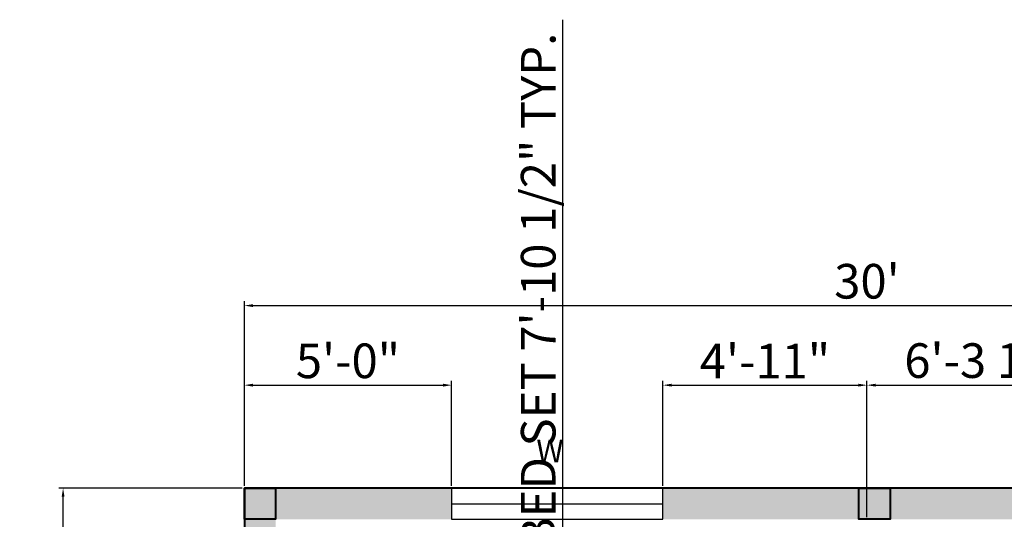
# Model space of a CAD drawing. Units: inches. Extents: x 1628 to 2197, y 2073 to 2736.
# Tile 2 of 3: x 1628 to 1913, y 2592 to 2736. Entities that reach past the tile are written whole.
import ezdxf

# ---------------------------------------------------------------- set-up
doc = ezdxf.new("R2010")
doc.units = ezdxf.units.IN
for name, color, linetype, lineweight in [('A-ANNO-DIMS', 2, 'Continuous', 18), ('A-ANNO-IDEN', 7, 'Continuous', 18), ('A-COLS', 7, 'Continuous', 40), ('A-COLS-PATT', 8, 'Continuous', 13), ('A-WALL-PATT', 152, 'Continuous', 13), ('wall', 151, 'Continuous', 40), ('window', 20, 'Continuous', 25)]:
    doc.layers.add(name, color=color, linetype=linetype, lineweight=lineweight)
doc.styles.get("Standard").update_dxf_attribs({"font": 'arial.ttf'})
doc.dimstyles.new('ISO-25', dxfattribs={"dimtxt": 10, "dimasz": 2.5, "dimexe": 1.25, "dimexo": 0.625, "dimtad": 1, "dimdec": 0, "dimlunit": 4, "dimtxsty": 'Standard', "dimcen": 2.5, "dimadec": 0, "dimazin": 0, "dimtfac": 1, "dimtdec": 0, "dimtmove": 0, "dimatfit": 3, "dimfxl": 1, "dimarcsym": 0})

# ---------------------------------------------------------------- blocks, each defined once
blk = doc.blocks.new('*D5')
at = {"layer": 'A-ANNO-DIMS', "color": 0, "lineweight": -2, "transparency": 16777216}
for p, q in [((1693.110896843685, 2601.327398616903), (1693.110896843685, 2654.686150997897)), ((1695.610896843685, 2653.436150997897), (2050.610896843686, 2653.436150997897)), ((2053.110896843686, 2601.327398616903), (2053.110896843686, 2654.686150997897))]:
    blk.add_line(p, q, dxfattribs=at)
at = {"layer": 'A-ANNO-DIMS', "color": 0, "transparency": 16777216}
for points in [[(1695.610896843685, 2653.852817664564), (1695.610896843685, 2653.019484331231), (1693.110896843685, 2653.436150997897)], [(2050.610896843686, 2653.852817664564), (2050.610896843686, 2653.019484331231), (2053.110896843686, 2653.436150997897)]]:
    blk.add_solid(points, dxfattribs=at)
at = {"layer": 'Defpoints', "color": 0, "transparency": 16777216}
for p in [(2053.110896843686, 2653.436150997897), (1693.110896843685, 2600.702398616903), (2053.110896843686, 2600.702398616903)]:
    blk.add_point(p, dxfattribs=at)
at = {"layer": 'A-ANNO-DIMS', "color": 0, "transparency": 16777216, "insert": (1873.110896843686, 2659.170291516315), "char_height": 10, "attachment_point": 5}
blk.add_mtext("30'", dxfattribs=at)
blk = doc.blocks.new('*D6')
at = {"layer": 'A-ANNO-DIMS', "color": 0, "lineweight": -2, "transparency": 16777216}
for p, q in [((1692.485896843686, 2600.702398616904), (1639.445355811252, 2600.702398616904)), ((1640.695355811253, 2123.202398616904), (1640.695355811252, 2598.202398616904)), ((1692.485896843686, 2120.702398616904), (1639.445355811253, 2120.702398616904))]:
    blk.add_line(p, q, dxfattribs=at)
at = {"layer": 'A-ANNO-DIMS', "color": 0, "transparency": 16777216}
for points in [[(1640.278689144586, 2598.202398616904), (1641.112022477919, 2598.202398616904), (1640.695355811252, 2600.702398616904)], [(1640.278689144586, 2123.202398616904), (1641.112022477919, 2123.202398616904), (1640.695355811253, 2120.702398616904)]]:
    blk.add_solid(points, dxfattribs=at)
at = {"layer": 'Defpoints', "color": 0, "transparency": 16777216}
for p in [(1640.695355811252, 2600.702398616904), (1693.110896843687, 2600.702398616904), (1693.110896843687, 2120.702398616904)]:
    blk.add_point(p, dxfattribs=at)
at = {"layer": 'A-ANNO-DIMS', "color": 0, "transparency": 16777216, "insert": (1634.964625934036, 2360.702398616903), "char_height": 10, "attachment_point": 5, "rotation": 90}
blk.add_mtext("40'", dxfattribs=at)
blk = doc.blocks.new('WINDOW-61IN')
blk.add_line((-0.0003684333103138, 4.500398616903112), (61.10273973038352, 4.500398616903112))
blk.add_lwpolyline([(-0.0003684333103138, 0.0003986169031123), (61.10273973038352, 0.0003986169031123), (61.10273973038352, 9.000398616903112), (-0.0003684333103138, 9.000398616903112)], close=True)
blk = doc.blocks.new('COLUMN-9X9')
blk.add_lwpolyline([(-0.0001031563144807, 9.000398616903112), (8.99989684368552, 9.000398616903112), (8.99989684368552, 0.0003986169031123), (-0.0001031563144807, 0.0003986169031123)], close=True)
blk = doc.blocks.new('*D19')
at = {"layer": 'A-ANNO-DIMS', "color": 0, "lineweight": -2, "transparency": 16777216}
for p, q in [((1785.152754647198, 2577.035625777927), (1785.152754647198, 2736.024370661965)), ((1771.578393576364, 2577.035625777927), (1786.402754647198, 2577.035625777927)), ((1785.152754647198, 2484.873218639036), (1785.152754647198, 2574.535625777927)), ((1771.578393576364, 2482.373218639037), (1786.402754647198, 2482.373218639037))]:
    blk.add_line(p, q, dxfattribs=at)
at = {"layer": 'A-ANNO-DIMS', "color": 0, "transparency": 16777216}
for points in [[(1784.736087980531, 2574.535625777927), (1785.569421313865, 2574.535625777927), (1785.152754647198, 2577.035625777927)], [(1784.736087980532, 2484.873218639036), (1785.569421313865, 2484.873218639036), (1785.152754647198, 2482.373218639037)]]:
    blk.add_solid(points, dxfattribs=at)
at = {"layer": 'Defpoints', "color": 0, "transparency": 16777216}
for p in [(1770.953393576364, 2577.035625777927), (1785.152754647198, 2577.035625777927), (1770.953393576364, 2482.373218639037)]:
    blk.add_point(p, dxfattribs=at)
at = {"layer": 'A-ANNO-DIMS', "color": 0, "transparency": 16777216, "insert": (1779.357222587171, 2657.779998219945), "char_height": 10, "attachment_point": 5, "rotation": 90}
blk.add_mtext('BED SET 7\'-10 1/2" TYP.', dxfattribs=at)
blk = doc.blocks.new('*D25')
at = {"layer": 'A-ANNO-DIMS', "color": 0, "lineweight": -2, "transparency": 16777216}
for p, q in [((1693.110897, 2601.327399), (1693.110897, 2631.702399)), ((1695.610897, 2630.452399), (1750.513632, 2630.452399)), ((1753.013632, 2601.327399), (1753.013632, 2631.702399))]:
    blk.add_line(p, q, dxfattribs=at)
at = {"layer": 'A-ANNO-DIMS', "color": 0, "transparency": 16777216}
for points in [[(1695.610897, 2630.869065666666), (1695.610897, 2630.035732333333), (1693.110897, 2630.452399)], [(1750.513632, 2630.869065666666), (1750.513632, 2630.035732333333), (1753.013632, 2630.452399)]]:
    blk.add_solid(points, dxfattribs=at)
at = {"layer": 'Defpoints', "color": 0, "transparency": 16777216}
for p in [(1753.013632, 2630.452399), (1693.110897, 2600.702399), (1753.013632, 2600.702399)]:
    blk.add_point(p, dxfattribs=at)
at = {"layer": 'A-ANNO-DIMS', "color": 0, "transparency": 16777216, "insert": (1723.0622645, 2636.183128877217), "char_height": 10, "attachment_point": 5}
blk.add_mtext('5\'-0"', dxfattribs=at)
blk = doc.blocks.new('*D26')
at = {"layer": 'A-ANNO-DIMS', "color": 0, "lineweight": -2, "transparency": 16777216}
for p, q in [((1814.11674, 2601.327399), (1814.11674, 2631.702399)), ((1816.61674, 2630.452399), (1870.610897, 2630.452399)), ((1873.110897, 2592.327399), (1873.110897, 2631.702399))]:
    blk.add_line(p, q, dxfattribs=at)
at = {"layer": 'A-ANNO-DIMS', "color": 0, "transparency": 16777216}
for points in [[(1816.61674, 2630.869065666666), (1816.61674, 2630.035732333333), (1814.11674, 2630.452399)], [(1870.610897, 2630.869065666666), (1870.610897, 2630.035732333333), (1873.110897, 2630.452399)]]:
    blk.add_solid(points, dxfattribs=at)
at = {"layer": 'Defpoints', "color": 0, "transparency": 16777216}
for p in [(1873.110897, 2630.452399), (1814.11674, 2600.702399), (1873.110897, 2591.702399)]:
    blk.add_point(p, dxfattribs=at)
at = {"layer": 'A-ANNO-DIMS', "color": 0, "transparency": 16777216, "insert": (1843.6138185, 2636.097862847203), "char_height": 10, "attachment_point": 5}
blk.add_mtext('4\'-11"', dxfattribs=at)
blk = doc.blocks.new('*D27')
at = {"layer": 'A-ANNO-DIMS', "color": 0, "lineweight": -2, "transparency": 16777216}
for p, q in [((1873.110897, 2592.327399), (1873.110897, 2631.702399)), ((1875.610897, 2630.452399), (1945.868746, 2630.452399)), ((1948.368746, 2601.327399), (1948.368746, 2631.702399))]:
    blk.add_line(p, q, dxfattribs=at)
at = {"layer": 'A-ANNO-DIMS', "color": 0, "transparency": 16777216}
for points in [[(1875.610897, 2630.869065666666), (1875.610897, 2630.035732333333), (1873.110897, 2630.452399)], [(1945.868746, 2630.869065666666), (1945.868746, 2630.035732333333), (1948.368746, 2630.452399)]]:
    blk.add_solid(points, dxfattribs=at)
at = {"layer": 'Defpoints', "color": 0, "transparency": 16777216}
for p in [(1948.368746, 2630.452399), (1948.368746, 2600.702399), (1873.110897, 2591.702399)]:
    blk.add_point(p, dxfattribs=at)
at = {"layer": 'A-ANNO-DIMS', "color": 0, "transparency": 16777216, "insert": (1910.7398215, 2636.251341701228), "char_height": 10, "attachment_point": 5}
blk.add_mtext('6\'-3 1/2"', dxfattribs=at)

msp = doc.modelspace()

# ---------------------------------------------------------------- hatches: boundary and pattern name
at = {"layer": 'A-COLS-PATT'}
h = msp.add_hatch(color=256, dxfattribs=at)
h.dxf.hatch_style = 1
h.paths.add_polyline_path([(1702.110896843685, 2600.702398616903), (1693.110896843685, 2600.702398616903), (1693.110896843685, 2591.702398616904), (1702.110896843685, 2591.702398616904)])
h.paths.add_polyline_path([(1879.789544656754, 2600.702398616903), (1870.789544656754, 2600.702398616903), (1870.789544656754, 2591.702398616904), (1879.789544656754, 2591.702398616904)])
h.paths.add_polyline_path([(2053.110896843686, 2600.702398616903), (2044.110896843686, 2600.702398616903), (2044.110896843686, 2591.702398616904), (2053.110896843686, 2591.702398616904)])
h.paths.add_polyline_path([(1702.110896843685, 2395.202398616904), (1693.110896843685, 2395.202398616904), (1693.110896843685, 2386.202398616903), (1702.110896843685, 2386.202398616903)])
h.paths.add_polyline_path([(1826.610896843686, 2395.202398616904), (1817.610896843685, 2395.202398616904), (1817.610896843685, 2386.202398616903), (1826.610896843686, 2386.202398616903)])
h.paths.add_polyline_path([(1702.110896843685, 2459.702398616903), (1693.110896843685, 2459.702398616903), (1693.110896843685, 2450.702398616904), (1702.110896843685, 2450.702398616904)])
h.paths.add_polyline_path([(2053.110896843686, 2459.702398616903), (2044.110896843686, 2459.702398616903), (2044.110896843686, 2455.202398616903), (2053.110896843686, 2455.202398616903)])
h.paths.add_polyline_path([(2053.110896843686, 2455.202398616903), (2044.110896843686, 2455.202398616903), (2044.110896843686, 2451.940390996), (2053.110896843686, 2451.940390996)])
h.paths.add_polyline_path([(2053.110896843686, 2460.940390996), (2044.110896843686, 2460.940390996), (2044.110896843686, 2459.702398616903), (2053.110896843686, 2459.702398616903)])
h.paths.add_polyline_path([(2053.110896843686, 2390.990533735672), (2044.110896843686, 2390.990533735672), (2044.110896843686, 2381.990533735671), (2053.110896843686, 2381.990533735671)])
h.paths.add_polyline_path([(2053.110896843686, 2322.517334083322), (2044.110896843686, 2322.517334083322), (2044.110896843686, 2313.517334083321), (2053.110896843686, 2313.517334083321)])
h.paths.add_polyline_path([(1702.110896843685, 2294.702398616903), (1693.110896843685, 2294.702398616903), (1693.110896843685, 2285.702398616903), (1702.110896843685, 2285.702398616903)])
h.paths.add_polyline_path([(1702.110896843685, 2129.702398616903), (1693.110896843685, 2129.702398616903), (1693.110896843685, 2120.702398616904), (1702.110896843685, 2120.702398616904)])
h.paths.add_polyline_path([(1831.350600622014, 2129.702398616903), (1822.350600622014, 2129.702398616903), (1822.350600622014, 2120.702398616904), (1831.350600622014, 2120.702398616904)])
h.paths.add_polyline_path([(1883.720266620277, 2129.702398616903), (1874.720266620277, 2129.702398616903), (1874.720266620277, 2120.702398616904), (1883.720266620277, 2120.702398616904)])
h.paths.add_polyline_path([(2053.110896843686, 2129.702398616903), (2044.110896843686, 2129.702398616903), (2044.110896843686, 2120.702398616904), (2053.110896843686, 2120.702398616904)])
at = {"layer": 'A-WALL-PATT'}
h = msp.add_hatch(color=256, dxfattribs=at)
h.dxf.hatch_style = 1
h.paths.add_polyline_path([(1753.013631566689, 2600.702398616903), (1702.110896843685, 2600.702398616903), (1702.110896843685, 2591.702398616904), (1753.013631566689, 2591.702398616904)])
h.paths.add_polyline_path([(1870.789544656754, 2600.702398616903), (1814.116739730383, 2600.702398616903), (1814.116739730383, 2591.702398616904), (1870.789544656754, 2591.702398616904)])
h.paths.add_polyline_path([(1948.368746460448, 2600.702398616903), (1879.789544656754, 2600.702398616903), (1879.789544656754, 2591.702398616904), (1909.320134716665, 2591.702398616904), (1948.368746460448, 2591.702398616904)])
h.paths.add_polyline_path([(2044.110896843686, 2600.702398616903), (2009.471854624142, 2600.702398616903), (2009.471854624142, 2591.702398616904), (2044.110896843686, 2591.702398616904)])
h.paths.add_polyline_path([(2053.110896843686, 2591.702398616904), (2044.110896843686, 2591.702398616904), (2044.110896843686, 2550.072421842385), (2053.110896843686, 2550.072421842385)])
h.paths.add_polyline_path([(1702.110896843685, 2591.702398616904), (1693.110896843685, 2591.702398616904), (1693.110896843685, 2549.953217094844), (1702.110896843685, 2549.953217094844)])
h.paths.add_polyline_path([(1702.110896843685, 2488.85010893115), (1693.110896843685, 2488.85010893115), (1693.110896843685, 2459.702398616903), (1702.110896843685, 2459.702398616903)])
h.paths.add_polyline_path([(1828.052739298115, 2459.702398616904), (1702.110896843685, 2459.702398616903), (1702.110896843685, 2455.202398616903), (1733.607219099031, 2455.202398616903), (1792.110896843686, 2455.202398616903), (1828.052739298115, 2455.202398616904)])
h.paths.add_polyline_path([(1885.432437777228, 2459.702398616904), (1868.052739298114, 2459.702398616904), (1868.052739298114, 2455.202398616904), (1885.432437777228, 2455.202398616904)])
h.paths.add_polyline_path([(2053.110896843686, 2488.969313678691), (2044.110896843686, 2488.969313678691), (2044.110896843686, 2474.676024548712), (2044.110896843686, 2460.940390996), (2053.110896843686, 2460.940390996)])
h.paths.add_polyline_path([(2053.110896843686, 2451.940390996), (2044.110896843686, 2451.940390996), (2044.110896843686, 2437.286361970541), (2053.110896843686, 2437.286361970541)])
h.paths.add_polyline_path([(2053.110896843686, 2414.882591286594), (2044.110896843686, 2414.882591286594), (2044.110896843686, 2390.990533735672), (2053.110896843686, 2390.990533735672)])
h.paths.add_polyline_path([(2044.110896843686, 2459.702398616903), (1925.432437777228, 2459.702398616904), (1925.432437777228, 2455.202398616904), (2044.110896843686, 2455.202398616903)])
h.paths.add_polyline_path([(2053.110896843686, 2381.990533735671), (2044.110896843686, 2381.990533735671), (2044.110896843686, 2322.517334083322), (2053.110896843686, 2322.517334083322)])
h.paths.add_polyline_path([(1919.510741842323, 2129.702398616903), (1883.720266620277, 2129.702398616903), (1883.720266620277, 2120.702398616904), (1919.510741842323, 2120.702398616904)])
h.paths.add_polyline_path([(2044.110896843686, 2129.702398616903), (1980.613850006017, 2129.702398616903), (1980.613850006017, 2120.702398616904), (2044.110896843686, 2120.702398616904)])
h.paths.add_polyline_path([(2053.110896843686, 2207.91287215655), (2044.110896843686, 2207.91287215655), (2044.110896843686, 2129.702398616903), (2053.110896843686, 2129.702398616903)])
h.paths.add_polyline_path([(2053.110896843686, 2313.517334083321), (2044.110896843686, 2313.517334083321), (2044.110896843686, 2269.015980320244), (2053.110896843686, 2269.015980320244)])
h.paths.add_polyline_path([(1822.350600622014, 2129.702398616903), (1785.245011413373, 2129.702398616903), (1785.245011413373, 2120.702398616904), (1822.350600622014, 2120.702398616904)])
h.paths.add_polyline_path([(1724.14190324968, 2129.702398616903), (1702.110896843685, 2129.702398616903), (1702.110896843685, 2120.702398616904), (1724.14190324968, 2120.702398616904)])
h.paths.add_polyline_path([(1702.110896843685, 2168.735790533592), (1693.110896843685, 2168.735790533592), (1693.110896843685, 2129.702398616903), (1702.110896843685, 2129.702398616903)])
h.paths.add_polyline_path([(1702.110896843685, 2285.702398616903), (1693.110896843685, 2285.702398616903), (1693.110896843685, 2229.838898697286), (1702.110896843685, 2229.838898697286)])
h.paths.add_polyline_path([(1702.110896843685, 2317.649084771689), (1693.110896843685, 2317.649084771689), (1693.110896843685, 2294.702398616903), (1702.110896843685, 2294.702398616903)])
h.paths.add_polyline_path([(1702.110896843685, 2386.202398616903), (1693.110896843685, 2386.202398616903), (1693.110896843685, 2378.752192935383), (1702.110896843685, 2378.752192935383)])
h.paths.add_polyline_path([(2044.110896843686, 2389.202398616903), (1938.645521324226, 2389.202398616903), (1938.645521324226, 2384.702398616903), (2044.110896843686, 2384.702398616903)])
h.paths.add_polyline_path([(1817.610896843685, 2395.202398616904), (1782.074184939754, 2395.202398616904), (1702.110896843685, 2395.202398616904), (1702.110896843685, 2390.702398616904), (1796.610896843685, 2390.702398616904), (1817.610896843685, 2390.702398616904)])
h.paths.add_polyline_path([(1796.610896843685, 2397.266058985151), (1792.110896843686, 2397.266058985151), (1792.110896843686, 2395.202398616904), (1796.610896843685, 2395.202398616904)])
h.paths.add_polyline_path([(1826.610896843686, 2386.202398616903), (1822.110896843685, 2386.202398616903), (1822.110896843685, 2339.518036859306), (1826.610896843686, 2339.518036859306)])
h.paths.add_polyline_path([(1826.610896843686, 2299.518036859305), (1822.110896843685, 2299.518036859305), (1822.110896843685, 2294.702398616903), (1822.110896843685, 2290.202398616903), (1826.610896843686, 2290.202398616903)])
h.paths.add_polyline_path([(1826.610896843686, 2290.202398616903), (1822.110896843685, 2290.202398616903), (1822.110896843685, 2285.084292625677), (1826.610896843686, 2285.084292625677)])
h.paths.add_polyline_path([(1822.110896843685, 2294.702398616903), (1702.110896843685, 2294.702398616903), (1702.110896843685, 2290.202398616903), (1770.513086395585, 2290.202398616903), (1822.110896843685, 2290.202398616903)])
h.paths.add_polyline_path([(1693.110896843685, 2437.863608426093), (1702.110896843685, 2437.863608426093), (1702.110896843685, 2450.702398616904), (1693.110896843685, 2450.702398616904)])
h.paths.add_polyline_path([(1702.110896843685, 2410.599065766391), (1693.110896843685, 2410.599065766391), (1693.110896843685, 2395.202398616904), (1702.110896843685, 2395.202398616904)])

# ---------------------------------------------------------------- linework, layer by layer
at = {"layer": 'wall'}
msp.add_lwpolyline([(1873.22691280648, 2120.702398616904), (2053.110896843686, 2120.702398616904), (2053.110896843686, 2600.702398616903), (1693.110896843685, 2600.702398616903), (1693.110896843685, 2120.702398616904), (1833.22691280648, 2120.702398616904)], dxfattribs=at)

# ---------------------------------------------------------------- block references
at = {"layer": 'A-COLS'}
for p in [(1693.111, 2591.702000000001), (1870.789647813069, 2591.702000000001)]:
    msp.add_blockref('COLUMN-9X9', p, dxfattribs=at)
at = {"layer": 'window'}
msp.add_blockref('WINDOW-61IN', (1753.014, 2591.702000000001), dxfattribs=at)

# ---------------------------------------------------------------- texts
at = {"layer": 'A-ANNO-IDEN', "insert": (1777.521270211575, 2614.676422773392), "char_height": 6.548575105434164, "attachment_point": 1}
msp.add_mtext_dynamic_manual_height_columns('W', width=86.8171032748999, gutter_width=32.74287552717082, heights=[0], dxfattribs=at)

# ---------------------------------------------------------------- dimensions: what is measured, and where the dimension line sits
at = {"layer": 'A-ANNO-DIMS'}
dim = msp.add_linear_dim(base=(1785.152754647198, 2577.035625777927), p1=(1770.953393576363, 2482.373218639035), p2=(1770.953393576363, 2577.035625777926), angle=90, text='BED SET <> TYP.', dimstyle='ISO-25', override={"dimdec": 1, "dimlfac": 1, "dimrnd": 0, "dimzin": 1, "dimdsep": 46, "dimlunit": 4, "dimfrac": 2}, dxfattribs=at)
dim.commit()
dim.dimension.update_dxf_attribs({"geometry": '*D19', "text_midpoint": (1779.357222587171, 2657.779998219945)})
for base, p1, p2, override, picture, middle in [((2053.110896843686, 2653.436150997897), (1693.110896843685, 2600.702398616903), (2053.110896843686, 2600.702398616903), {"dimclrd": 0, "dimclre": 0, "dimclrt": 0}, '*D5', (1873.110896843686, 2659.170291516315)), ((1948.368746, 2630.452399), (1873.110897, 2591.702399), (1948.368746, 2600.702399), {"dimdec": 1, "dimlfac": 1, "dimrnd": 0, "dimzin": 1, "dimdsep": 46, "dimlunit": 4, "dimfrac": 2}, '*D27', (1910.7398215, 2636.251341701228)), ((1753.013632, 2630.452399), (1693.110897, 2600.702399), (1753.013632, 2600.702399), {"dimdec": 1, "dimlfac": 1, "dimrnd": 0, "dimzin": 1, "dimdsep": 46, "dimlunit": 4, "dimfrac": 2}, '*D25', (1723.0622645, 2636.183128877217)), ((1873.110897, 2630.452399), (1814.11674, 2600.702399), (1873.110897, 2591.702399), {"dimdec": 1, "dimlfac": 1, "dimrnd": 0, "dimzin": 1, "dimdsep": 46, "dimlunit": 4, "dimfrac": 2}, '*D26', (1843.6138185, 2636.097862847203))]:
    dim = msp.add_linear_dim(base=base, p1=p1, p2=p2, dimstyle='ISO-25', override=override, dxfattribs=at)
    dim.commit()
    dim.dimension.update_dxf_attribs({"geometry": picture, "text_midpoint": middle})
dim = msp.add_linear_dim(base=(1640.695355811252, 2600.702398616904), p1=(1693.110896843685, 2120.702398616904), p2=(1693.110896843685, 2600.702398616903), angle=90, dimstyle='ISO-25', override={"dimclrd": 0, "dimclre": 0, "dimclrt": 0}, dxfattribs=at)
dim.commit()
dim.dimension.update_dxf_attribs({"geometry": '*D6', "text_midpoint": (1634.964625934036, 2360.702398616903)})

doc.saveas('drawing.dxf')
